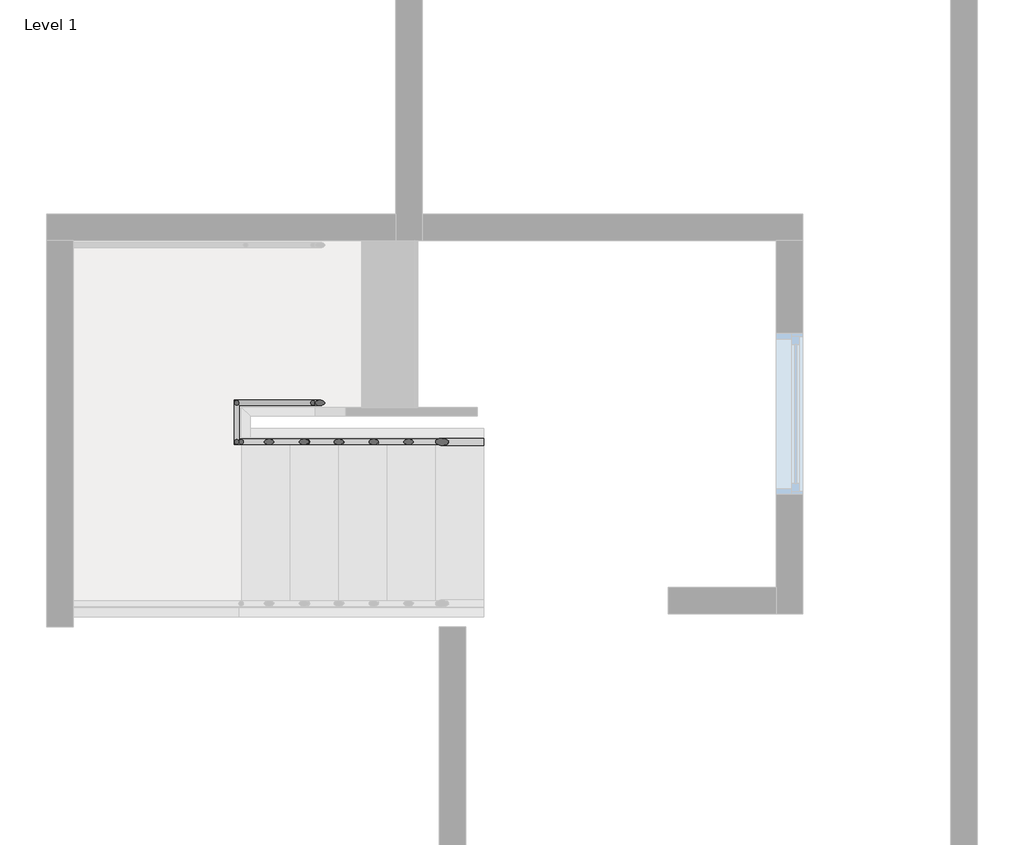
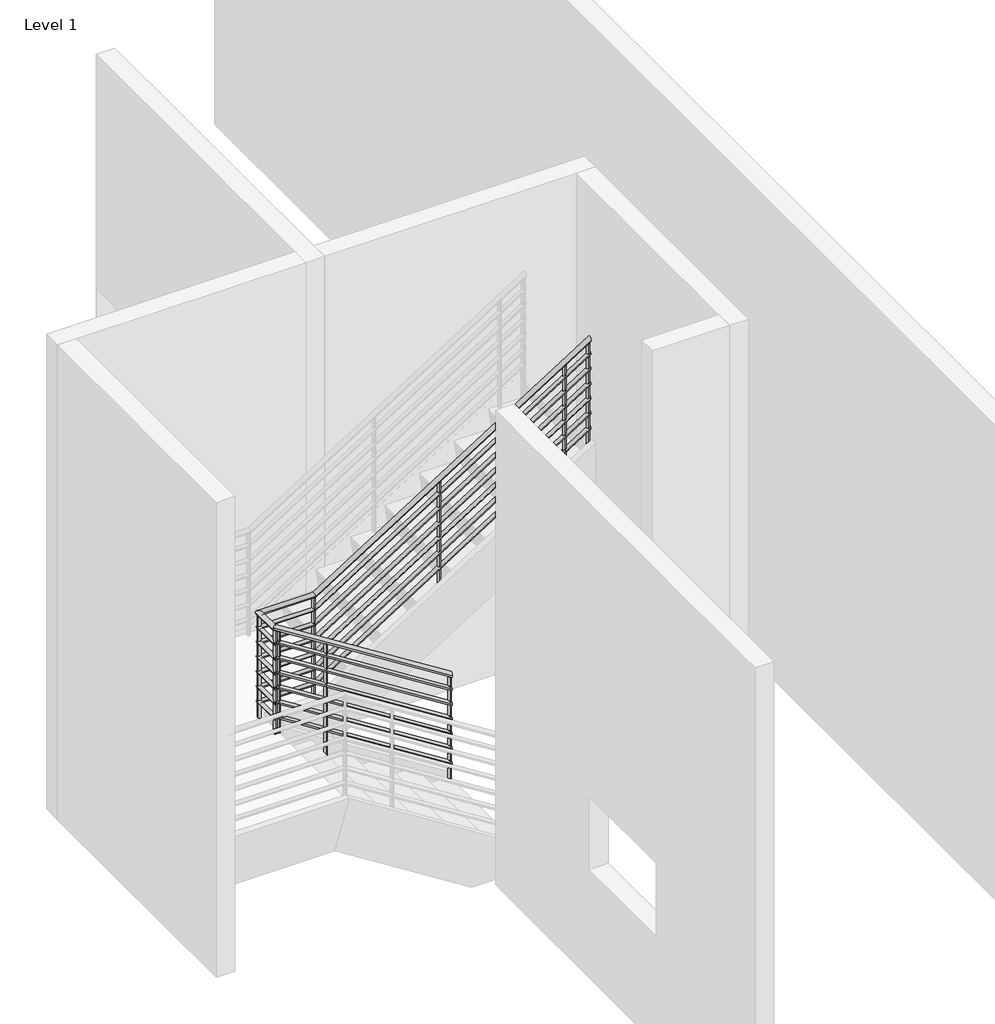
# One storey, part 3 of 4: 1 railing.
"""IFC4 building model written with IfcOpenShell, lengths in millimetres."""

from ifc_helpers import new_model, si_unit, point, frame, frame_2d, origin, place, context, project, spatial, circle_curve, ellipse_curve, trimmed, segment, composite_curve, outline, extrude, element, save
from ifc_brep_helpers import plane_surface, cylinder_surface, advanced_brep

model = new_model("IFC4")

# Units and contexts
model_context = context("Model", 3, world=origin())
ifc_project = project(units=[si_unit("LENGTHUNIT", "METRE", prefix="MILLI")], contexts=[model_context])

# Site, building, storey
site = spatial("IfcSite", under=ifc_project)
building = spatial("IfcBuilding", under=site)
storey = spatial("IfcBuildingStorey", under=building, Name="Level 1", Elevation=0.0)

# Railing
placement = place(None, origin())
element("IfcRailing", 1, ObjectType="900mm Pipe", at=placement, inside=storey, context=model_context, shape_type="SolidModel", body=[
    advanced_brep(
    [(-539.0915237, 1805.4567276, 1050.2491997), (-539.0915237, 1765.4567276, 1050.2491997), (-1933.2780119, 1805.4567276, 1931.9481645), (-1967.0848612, 1765.4567276, 1953.3279902)],
    [
        (0, 1, ellipse_curve(frame((-539.0915237, 1785.4567276, 1050.2491997), z_axis=(1.0, 0.0, 0.0), x_axis=(0.0, 0.0, -1.0)), 23.6638438, 20.0)),
        (1, 0, ellipse_curve(frame((-539.0915237, 1785.4567276, 1050.2491997), z_axis=(1.0, 0.0, 0.0), x_axis=(0.0, 0.0, -1.0)), 23.6638438, 20.0)),
        (2, 3, ellipse_curve(frame((-1950.1814365, 1785.4567276, 1942.6380773), z_axis=(-0.5976263089853376, 0.7071067811865505, 0.37794549184843795), x_axis=(0.597626308985345, 0.7071067811865448, -0.37794549184843707)), 28.2842712, 20.0)),
        (3, 2, ellipse_curve(frame((-1950.1814365, 1785.4567276, 1942.6380773), z_axis=(-0.5976263089853376, 0.7071067811865505, 0.37794549184843795), x_axis=(0.597626308985345, 0.7071067811865448, -0.37794549184843707)), 28.2842712, 20.0)),
        (0, 2),
        (3, 1),
    ],
    [
        plane_surface(frame((-539.0915237, 1785.4567276, 1073.9130435), z_axis=(1.0, 0.0, 0.0), x_axis=(0.0, -1.0, 0.0))),
        plane_surface(frame((-1939.4915237, 1785.4567276, 1959.541502), z_axis=(-0.5976263089853376, 0.7071067811865505, 0.37794549184843795), x_axis=(0.8017747781070204, 0.5270627453469413, 0.281712739610376))),
        cylinder_surface(frame((-549.7814365, 1785.4567276, 1057.0096189), z_axis=(0.8451712313980436, 0.0, -0.5344956404098304), x_axis=(0.0, -1.0, 0.0)), 20.0),
    ],
    [
        (0, [[1, 2]]),
        (1, [[3, 4]]),
        (2, [[-1, 5, -4, 6]]),
        (2, [[-2, -6, -3, -5]]),
    ],
),
    advanced_brep(
    [(-1919.4915237, 1813.050065, 1923.4782609), (-1959.4915237, 1779.2432158, 1923.4782609), (-1919.4915237, 1986.3593033, 1923.4782609), (-1959.4915237, 2026.3593033, 1923.4782609), (-1501.6762623, 1986.3593033, 1923.4782609), (-1501.6762623, 2026.3593033, 1923.4782609), (692.5302847, 1986.3593033, 3311.1187649), (692.5302847, 2026.3593033, 3311.1187649)],
    [
        (0, 1, ellipse_curve(frame((-1939.4915237, 1796.1466404, 1923.4782609), z_axis=(0.5976263089853376, -0.7071067811865505, -0.37794549184843795), x_axis=(-0.5976263089853452, -0.7071067811865446, 0.37794549184843695)), 28.2842712, 20.0)),
        (1, 0, ellipse_curve(frame((-1939.4915237, 1796.1466404, 1923.4782609), z_axis=(0.5976263089853376, -0.7071067811865505, -0.37794549184843795), x_axis=(-0.5976263089853452, -0.7071067811865446, 0.37794549184843695)), 28.2842712, 20.0)),
        (0, 2),
        (2, 3, ellipse_curve(frame((-1939.4915237, 2006.3593033, 1923.4782609), z_axis=(-0.7071067811865511, -0.707106781186544, 0.0), x_axis=(0.7071067811865441, -0.707106781186551, 0.0)), 28.2842712, 20.0)),
        (3, 1),
        (3, 2, ellipse_curve(frame((-1939.4915237, 2006.3593033, 1923.4782609), z_axis=(-0.7071067811865511, -0.707106781186544, 0.0), x_axis=(0.7071067811865441, -0.707106781186551, 0.0)), 28.2842712, 20.0)),
        (2, 4),
        (4, 5, ellipse_curve(frame((-1501.6762623, 2006.3593033, 1923.4782609), z_axis=(-0.9605132043335073, 0.0, -0.27823440531497556), x_axis=(-0.2782344053149757, 0.0, 0.9605132043335073)), 20.822202, 20.0)),
        (5, 3),
        (5, 4, ellipse_curve(frame((-1501.6762623, 2006.3593033, 1923.4782609), z_axis=(-0.9605132043335073, 0.0, -0.27823440531497556), x_axis=(-0.2782344053149757, 0.0, 0.9605132043335073)), 20.822202, 20.0)),
        (6, 7, ellipse_curve(frame((692.5302847, 2006.3593033, 3311.1187649), z_axis=(1.0, 0.0, 0.0), x_axis=(0.0, 0.0, -1.0)), 23.6638438, 20.0)),
        (7, 6, ellipse_curve(frame((692.5302847, 2006.3593033, 3311.1187649), z_axis=(1.0, 0.0, 0.0), x_axis=(0.0, 0.0, -1.0)), 23.6638438, 20.0)),
        (4, 6),
        (7, 5),
    ],
    [
        plane_surface(frame((-1939.4915237, 1785.4567276, 1943.4782609), z_axis=(0.5976263089853376, -0.7071067811865505, -0.37794549184843795), x_axis=(0.8017747781070204, 0.5270627453469413, 0.281712739610376))),
        cylinder_surface(frame((-1939.4915237, 1785.4567276, 1923.4782609), z_axis=(0.0, -1.0, 0.0), x_axis=(-1.0, 0.0, 0.0)), 20.0),
        cylinder_surface(frame((-1939.4915237, 2006.3593033, 1923.4782609), z_axis=(-1.0, 0.0, 0.0), x_axis=(0.0, 1.0, 0.0)), 20.0),
        plane_surface(frame((692.5302847, 2006.3593033, 3334.7826087), z_axis=(1.0, 0.0, 0.0), x_axis=(0.0, 1.0, 0.0))),
        cylinder_surface(frame((-1496.7798025, 2006.3593033, 1926.5748362), z_axis=(-0.8451712313980438, 0.0, -0.5344956404098301), x_axis=(0.0, 1.0, 0.0)), 20.0),
    ],
    [
        (0, [[1, 2]]),
        (1, [[-1, 3, 4, 5]]),
        (1, [[-2, -5, 6, -3]]),
        (2, [[-4, 7, 8, 9]]),
        (2, [[-6, -9, 10, -7]]),
        (3, [[11, 12]]),
        (4, [[-8, 13, -12, 14]]),
        (4, [[-10, -14, -11, -13]]),
    ],
),
    advanced_brep(
    [(-539.0915237, 1770.4567276, 931.1651606), (-539.0915237, 1800.4567276, 931.1651606), (-1918.4366135, 1770.4567276, 1803.4782609), (-1918.4366135, 1800.4567276, 1803.4782609), (-1954.4915237, 1770.4567276, 1803.4782609), (-1924.4915237, 1800.4567276, 1803.4782609), (-1954.4915237, 2021.3593033, 1803.4782609), (-1924.4915237, 1991.3593033, 1803.4782609), (-1503.1246256, 2021.3593033, 1803.4782609), (-1503.1246256, 1991.3593033, 1803.4782609), (692.5302847, 2021.3593033, 3192.0347258), (692.5302847, 1991.3593033, 3192.0347258)],
    [
        (0, 1, ellipse_curve(frame((-539.0915237, 1785.4567276, 931.1651606), z_axis=(1.0, 0.0, 0.0), x_axis=(0.0, 0.0, -1.0)), 17.7478828, 15.0)),
        (1, 0, ellipse_curve(frame((-539.0915237, 1785.4567276, 931.1651606), z_axis=(1.0, 0.0, 0.0), x_axis=(0.0, 0.0, -1.0)), 17.7478828, 15.0)),
        (0, 2),
        (2, 3, ellipse_curve(frame((-1918.4366135, 1785.4567276, 1803.4782609), z_axis=(0.9605132043335073, 0.0, -0.27823440531497584), x_axis=(-0.2782344053149764, 0.0, -0.9605132043335071)), 15.6166515, 15.0)),
        (3, 1),
        (3, 2, ellipse_curve(frame((-1918.4366135, 1785.4567276, 1803.4782609), z_axis=(0.9605132043335073, 0.0, -0.27823440531497584), x_axis=(-0.2782344053149764, 0.0, -0.9605132043335071)), 15.6166515, 15.0)),
        (2, 4),
        (4, 5, ellipse_curve(frame((-1939.4915237, 1785.4567276, 1803.4782609), z_axis=(0.7071067811865441, -0.7071067811865509, 0.0), x_axis=(0.707106781186551, 0.7071067811865441, 0.0)), 21.2132034, 15.0)),
        (5, 3),
        (5, 4, ellipse_curve(frame((-1939.4915237, 1785.4567276, 1803.4782609), z_axis=(0.7071067811865441, -0.7071067811865509, 0.0), x_axis=(0.707106781186551, 0.7071067811865441, 0.0)), 21.2132034, 15.0)),
        (4, 6),
        (6, 7, ellipse_curve(frame((-1939.4915237, 2006.3593033, 1803.4782609), z_axis=(-0.7071067811865511, -0.707106781186544, 0.0), x_axis=(0.7071067811865441, -0.707106781186551, 0.0)), 21.2132034, 15.0)),
        (7, 5),
        (7, 6, ellipse_curve(frame((-1939.4915237, 2006.3593033, 1803.4782609), z_axis=(-0.7071067811865511, -0.707106781186544, 0.0), x_axis=(0.7071067811865441, -0.707106781186551, 0.0)), 21.2132034, 15.0)),
        (6, 8),
        (8, 9, ellipse_curve(frame((-1503.1246256, 2006.3593033, 1803.4782609), z_axis=(-0.9605132043335072, 0.0, -0.2782344053149756), x_axis=(-0.27823440531497606, 0.0, 0.9605132043335073)), 15.6166515, 15.0)),
        (9, 7),
        (9, 8, ellipse_curve(frame((-1503.1246256, 2006.3593033, 1803.4782609), z_axis=(-0.9605132043335072, 0.0, -0.2782344053149756), x_axis=(-0.27823440531497606, 0.0, 0.9605132043335073)), 15.6166515, 15.0)),
        (10, 11, ellipse_curve(frame((692.5302847, 2006.3593033, 3192.0347258), z_axis=(1.0, 0.0, 0.0), x_axis=(0.0, 0.0, -1.0)), 17.7478828, 15.0)),
        (11, 10, ellipse_curve(frame((692.5302847, 2006.3593033, 3192.0347258), z_axis=(1.0, 0.0, 0.0), x_axis=(0.0, 0.0, -1.0)), 17.7478828, 15.0)),
        (8, 10),
        (11, 9),
    ],
    [
        plane_surface(frame((-539.0915237, 1785.4567276, 948.9130435), z_axis=(1.0, 0.0, 0.0), x_axis=(0.0, -1.0, 0.0))),
        cylinder_surface(frame((-547.1089583, 1785.4567276, 936.235475), z_axis=(0.8451712313980436, 0.0, -0.5344956404098303), x_axis=(0.0, 1.0, 0.0)), 15.0),
        cylinder_surface(frame((-1914.0915237, 1785.4567276, 1803.4782609), z_axis=(1.0, 0.0, 0.0), x_axis=(0.0, 1.0, 0.0)), 15.0),
        cylinder_surface(frame((-1939.4915237, 1785.4567276, 1803.4782609), z_axis=(0.0, -1.0, 0.0), x_axis=(1.0, 0.0, 0.0)), 15.0),
        cylinder_surface(frame((-1939.4915237, 2006.3593033, 1803.4782609), z_axis=(-1.0, 0.0, 0.0), x_axis=(0.0, -1.0, 0.0)), 15.0),
        plane_surface(frame((692.5302847, 2006.3593033, 3209.7826087), z_axis=(1.0, 0.0, 0.0), x_axis=(0.0, 1.0, 0.0))),
        cylinder_surface(frame((-1499.4522807, 2006.3593033, 1805.8006924), z_axis=(-0.8451712313980437, 0.0, -0.5344956404098301), x_axis=(0.0, -1.0, 0.0)), 15.0),
    ],
    [
        (0, [[1, 2]]),
        (1, [[-1, 3, 4, 5]]),
        (1, [[-2, -5, 6, -3]]),
        (2, [[-4, 7, 8, 9]]),
        (2, [[-6, -9, 10, -7]]),
        (3, [[-8, 11, 12, 13]]),
        (3, [[-10, -13, 14, -11]]),
        (4, [[-12, 15, 16, 17]]),
        (4, [[-14, -17, 18, -15]]),
        (5, [[19, 20]]),
        (6, [[-16, 21, -20, 22]]),
        (6, [[-18, -22, -19, -21]]),
    ],
),
    advanced_brep(
    [(-539.0915237, 1770.4567276, 806.1651606), (-539.0915237, 1800.4567276, 806.1651606), (-1918.4366135, 1770.4567276, 1678.4782609), (-1918.4366135, 1800.4567276, 1678.4782609), (-1954.4915237, 1770.4567276, 1678.4782609), (-1924.4915237, 1800.4567276, 1678.4782609), (-1954.4915237, 2021.3593033, 1678.4782609), (-1924.4915237, 1991.3593033, 1678.4782609), (-1503.1246256, 2021.3593033, 1678.4782609), (-1503.1246256, 1991.3593033, 1678.4782609), (692.5302847, 2021.3593033, 3067.0347258), (692.5302847, 1991.3593033, 3067.0347258)],
    [
        (0, 1, ellipse_curve(frame((-539.0915237, 1785.4567276, 806.1651606), z_axis=(1.0, 0.0, 0.0), x_axis=(0.0, 0.0, -1.0)), 17.7478828, 15.0)),
        (1, 0, ellipse_curve(frame((-539.0915237, 1785.4567276, 806.1651606), z_axis=(1.0, 0.0, 0.0), x_axis=(0.0, 0.0, -1.0)), 17.7478828, 15.0)),
        (0, 2),
        (2, 3, ellipse_curve(frame((-1918.4366135, 1785.4567276, 1678.4782609), z_axis=(0.9605132043335073, 0.0, -0.27823440531497584), x_axis=(-0.2782344053149764, 0.0, -0.9605132043335071)), 15.6166515, 15.0)),
        (3, 1),
        (3, 2, ellipse_curve(frame((-1918.4366135, 1785.4567276, 1678.4782609), z_axis=(0.9605132043335073, 0.0, -0.27823440531497584), x_axis=(-0.2782344053149764, 0.0, -0.9605132043335071)), 15.6166515, 15.0)),
        (2, 4),
        (4, 5, ellipse_curve(frame((-1939.4915237, 1785.4567276, 1678.4782609), z_axis=(0.7071067811865441, -0.7071067811865509, 0.0), x_axis=(0.707106781186551, 0.7071067811865441, 0.0)), 21.2132034, 15.0)),
        (5, 3),
        (5, 4, ellipse_curve(frame((-1939.4915237, 1785.4567276, 1678.4782609), z_axis=(0.7071067811865441, -0.7071067811865509, 0.0), x_axis=(0.707106781186551, 0.7071067811865441, 0.0)), 21.2132034, 15.0)),
        (4, 6),
        (6, 7, ellipse_curve(frame((-1939.4915237, 2006.3593033, 1678.4782609), z_axis=(-0.7071067811865511, -0.707106781186544, 0.0), x_axis=(0.7071067811865441, -0.707106781186551, 0.0)), 21.2132034, 15.0)),
        (7, 5),
        (7, 6, ellipse_curve(frame((-1939.4915237, 2006.3593033, 1678.4782609), z_axis=(-0.7071067811865511, -0.707106781186544, 0.0), x_axis=(0.7071067811865441, -0.707106781186551, 0.0)), 21.2132034, 15.0)),
        (6, 8),
        (8, 9, ellipse_curve(frame((-1503.1246256, 2006.3593033, 1678.4782609), z_axis=(-0.9605132043335073, 0.0, -0.2782344053149756), x_axis=(-0.2782344053149757, 0.0, 0.9605132043335073)), 15.6166515, 15.0)),
        (9, 7),
        (9, 8, ellipse_curve(frame((-1503.1246256, 2006.3593033, 1678.4782609), z_axis=(-0.9605132043335073, 0.0, -0.2782344053149756), x_axis=(-0.2782344053149757, 0.0, 0.9605132043335073)), 15.6166515, 15.0)),
        (10, 11, ellipse_curve(frame((692.5302847, 2006.3593033, 3067.0347258), z_axis=(1.0, 0.0, 0.0), x_axis=(0.0, 0.0, -1.0)), 17.7478828, 15.0)),
        (11, 10, ellipse_curve(frame((692.5302847, 2006.3593033, 3067.0347258), z_axis=(1.0, 0.0, 0.0), x_axis=(0.0, 0.0, -1.0)), 17.7478828, 15.0)),
        (8, 10),
        (11, 9),
    ],
    [
        plane_surface(frame((-539.0915237, 1785.4567276, 823.9130435), z_axis=(1.0, 0.0, 0.0), x_axis=(0.0, -1.0, 0.0))),
        cylinder_surface(frame((-547.1089583, 1785.4567276, 811.235475), z_axis=(0.8451712313980436, 0.0, -0.5344956404098303), x_axis=(0.0, 1.0, 0.0)), 15.0),
        cylinder_surface(frame((-1914.0915237, 1785.4567276, 1678.4782609), z_axis=(1.0, 0.0, 0.0), x_axis=(0.0, 1.0, 0.0)), 15.0),
        cylinder_surface(frame((-1939.4915237, 1785.4567276, 1678.4782609), z_axis=(0.0, -1.0, 0.0), x_axis=(1.0, 0.0, 0.0)), 15.0),
        cylinder_surface(frame((-1939.4915237, 2006.3593033, 1678.4782609), z_axis=(-1.0, 0.0, 0.0), x_axis=(0.0, -1.0, 0.0)), 15.0),
        plane_surface(frame((692.5302847, 2006.3593033, 3084.7826087), z_axis=(1.0, 0.0, 0.0), x_axis=(0.0, 1.0, 0.0))),
        cylinder_surface(frame((-1499.4522807, 2006.3593033, 1680.8006924), z_axis=(-0.8451712313980438, 0.0, -0.5344956404098301), x_axis=(0.0, -1.0, 0.0)), 15.0),
    ],
    [
        (0, [[1, 2]]),
        (1, [[-1, 3, 4, 5]]),
        (1, [[-2, -5, 6, -3]]),
        (2, [[-4, 7, 8, 9]]),
        (2, [[-6, -9, 10, -7]]),
        (3, [[-8, 11, 12, 13]]),
        (3, [[-10, -13, 14, -11]]),
        (4, [[-12, 15, 16, 17]]),
        (4, [[-14, -17, 18, -15]]),
        (5, [[19, 20]]),
        (6, [[-16, 21, -20, 22]]),
        (6, [[-18, -22, -19, -21]]),
    ],
),
    advanced_brep(
    [(-539.0915237, 1770.4567276, 681.1651606), (-539.0915237, 1800.4567276, 681.1651606), (-1918.4366135, 1770.4567276, 1553.4782609), (-1918.4366135, 1800.4567276, 1553.4782609), (-1954.4915237, 1770.4567276, 1553.4782609), (-1924.4915237, 1800.4567276, 1553.4782609), (-1954.4915237, 2021.3593033, 1553.4782609), (-1924.4915237, 1991.3593033, 1553.4782609), (-1503.1246256, 2021.3593033, 1553.4782609), (-1503.1246256, 1991.3593033, 1553.4782609), (692.5302847, 2021.3593033, 2942.0347258), (692.5302847, 1991.3593033, 2942.0347258)],
    [
        (0, 1, ellipse_curve(frame((-539.0915237, 1785.4567276, 681.1651606), z_axis=(1.0, 0.0, 0.0), x_axis=(0.0, 0.0, -1.0)), 17.7478828, 15.0)),
        (1, 0, ellipse_curve(frame((-539.0915237, 1785.4567276, 681.1651606), z_axis=(1.0, 0.0, 0.0), x_axis=(0.0, 0.0, -1.0)), 17.7478828, 15.0)),
        (0, 2),
        (2, 3, ellipse_curve(frame((-1918.4366135, 1785.4567276, 1553.4782609), z_axis=(0.9605132043335073, 0.0, -0.27823440531497584), x_axis=(-0.2782344053149764, 0.0, -0.9605132043335071)), 15.6166515, 15.0)),
        (3, 1),
        (3, 2, ellipse_curve(frame((-1918.4366135, 1785.4567276, 1553.4782609), z_axis=(0.9605132043335073, 0.0, -0.27823440531497584), x_axis=(-0.2782344053149764, 0.0, -0.9605132043335071)), 15.6166515, 15.0)),
        (2, 4),
        (4, 5, ellipse_curve(frame((-1939.4915237, 1785.4567276, 1553.4782609), z_axis=(0.7071067811865441, -0.7071067811865509, 0.0), x_axis=(0.707106781186551, 0.7071067811865441, 0.0)), 21.2132034, 15.0)),
        (5, 3),
        (5, 4, ellipse_curve(frame((-1939.4915237, 1785.4567276, 1553.4782609), z_axis=(0.7071067811865441, -0.7071067811865509, 0.0), x_axis=(0.707106781186551, 0.7071067811865441, 0.0)), 21.2132034, 15.0)),
        (4, 6),
        (6, 7, ellipse_curve(frame((-1939.4915237, 2006.3593033, 1553.4782609), z_axis=(-0.7071067811865511, -0.707106781186544, 0.0), x_axis=(0.7071067811865441, -0.707106781186551, 0.0)), 21.2132034, 15.0)),
        (7, 5),
        (7, 6, ellipse_curve(frame((-1939.4915237, 2006.3593033, 1553.4782609), z_axis=(-0.7071067811865511, -0.707106781186544, 0.0), x_axis=(0.7071067811865441, -0.707106781186551, 0.0)), 21.2132034, 15.0)),
        (6, 8),
        (8, 9, ellipse_curve(frame((-1503.1246256, 2006.3593033, 1553.4782609), z_axis=(-0.9605132043335073, 0.0, -0.2782344053149756), x_axis=(-0.2782344053149757, 0.0, 0.9605132043335073)), 15.6166515, 15.0)),
        (9, 7),
        (9, 8, ellipse_curve(frame((-1503.1246256, 2006.3593033, 1553.4782609), z_axis=(-0.9605132043335073, 0.0, -0.2782344053149756), x_axis=(-0.2782344053149757, 0.0, 0.9605132043335073)), 15.6166515, 15.0)),
        (10, 11, ellipse_curve(frame((692.5302847, 2006.3593033, 2942.0347258), z_axis=(1.0, 0.0, 0.0), x_axis=(0.0, 0.0, -1.0)), 17.7478828, 15.0)),
        (11, 10, ellipse_curve(frame((692.5302847, 2006.3593033, 2942.0347258), z_axis=(1.0, 0.0, 0.0), x_axis=(0.0, 0.0, -1.0)), 17.7478828, 15.0)),
        (8, 10),
        (11, 9),
    ],
    [
        plane_surface(frame((-539.0915237, 1785.4567276, 698.9130435), z_axis=(1.0, 0.0, 0.0), x_axis=(0.0, -1.0, 0.0))),
        cylinder_surface(frame((-547.1089583, 1785.4567276, 686.235475), z_axis=(0.8451712313980436, 0.0, -0.5344956404098303), x_axis=(0.0, 1.0, 0.0)), 15.0),
        cylinder_surface(frame((-1914.0915237, 1785.4567276, 1553.4782609), z_axis=(1.0, 0.0, 0.0), x_axis=(0.0, 1.0, 0.0)), 15.0),
        cylinder_surface(frame((-1939.4915237, 1785.4567276, 1553.4782609), z_axis=(0.0, -1.0, 0.0), x_axis=(1.0, 0.0, 0.0)), 15.0),
        cylinder_surface(frame((-1939.4915237, 2006.3593033, 1553.4782609), z_axis=(-1.0, 0.0, 0.0), x_axis=(0.0, -1.0, 0.0)), 15.0),
        plane_surface(frame((692.5302847, 2006.3593033, 2959.7826087), z_axis=(1.0, 0.0, 0.0), x_axis=(0.0, 1.0, 0.0))),
        cylinder_surface(frame((-1499.4522807, 2006.3593033, 1555.8006924), z_axis=(-0.8451712313980438, 0.0, -0.5344956404098301), x_axis=(0.0, -1.0, 0.0)), 15.0),
    ],
    [
        (0, [[1, 2]]),
        (1, [[-1, 3, 4, 5]]),
        (1, [[-2, -5, 6, -3]]),
        (2, [[-4, 7, 8, 9]]),
        (2, [[-6, -9, 10, -7]]),
        (3, [[-8, 11, 12, 13]]),
        (3, [[-10, -13, 14, -11]]),
        (4, [[-12, 15, 16, 17]]),
        (4, [[-14, -17, 18, -15]]),
        (5, [[19, 20]]),
        (6, [[-16, 21, -20, 22]]),
        (6, [[-18, -22, -19, -21]]),
    ],
),
    advanced_brep(
    [(-539.0915237, 1770.4567276, 556.1651606), (-539.0915237, 1800.4567276, 556.1651606), (-1918.4366135, 1770.4567276, 1428.4782609), (-1918.4366135, 1800.4567276, 1428.4782609), (-1954.4915237, 1770.4567276, 1428.4782609), (-1924.4915237, 1800.4567276, 1428.4782609), (-1954.4915237, 2021.3593033, 1428.4782609), (-1924.4915237, 1991.3593033, 1428.4782609), (-1503.1246256, 2021.3593033, 1428.4782609), (-1503.1246256, 1991.3593033, 1428.4782609), (692.5302847, 2021.3593033, 2817.0347258), (692.5302847, 1991.3593033, 2817.0347258)],
    [
        (0, 1, ellipse_curve(frame((-539.0915237, 1785.4567276, 556.1651606), z_axis=(1.0, 0.0, 0.0), x_axis=(0.0, 0.0, -1.0)), 17.7478828, 15.0)),
        (1, 0, ellipse_curve(frame((-539.0915237, 1785.4567276, 556.1651606), z_axis=(1.0, 0.0, 0.0), x_axis=(0.0, 0.0, -1.0)), 17.7478828, 15.0)),
        (0, 2),
        (2, 3, ellipse_curve(frame((-1918.4366135, 1785.4567276, 1428.4782609), z_axis=(0.9605132043335073, 0.0, -0.27823440531497584), x_axis=(-0.2782344053149764, 0.0, -0.9605132043335071)), 15.6166515, 15.0)),
        (3, 1),
        (3, 2, ellipse_curve(frame((-1918.4366135, 1785.4567276, 1428.4782609), z_axis=(0.9605132043335073, 0.0, -0.27823440531497584), x_axis=(-0.2782344053149764, 0.0, -0.9605132043335071)), 15.6166515, 15.0)),
        (2, 4),
        (4, 5, ellipse_curve(frame((-1939.4915237, 1785.4567276, 1428.4782609), z_axis=(0.7071067811865441, -0.7071067811865509, 0.0), x_axis=(0.707106781186551, 0.7071067811865441, 0.0)), 21.2132034, 15.0)),
        (5, 3),
        (5, 4, ellipse_curve(frame((-1939.4915237, 1785.4567276, 1428.4782609), z_axis=(0.7071067811865441, -0.7071067811865509, 0.0), x_axis=(0.707106781186551, 0.7071067811865441, 0.0)), 21.2132034, 15.0)),
        (4, 6),
        (6, 7, ellipse_curve(frame((-1939.4915237, 2006.3593033, 1428.4782609), z_axis=(-0.7071067811865511, -0.707106781186544, 0.0), x_axis=(0.7071067811865441, -0.707106781186551, 0.0)), 21.2132034, 15.0)),
        (7, 5),
        (7, 6, ellipse_curve(frame((-1939.4915237, 2006.3593033, 1428.4782609), z_axis=(-0.7071067811865511, -0.707106781186544, 0.0), x_axis=(0.7071067811865441, -0.707106781186551, 0.0)), 21.2132034, 15.0)),
        (6, 8),
        (8, 9, ellipse_curve(frame((-1503.1246256, 2006.3593033, 1428.4782609), z_axis=(-0.9605132043335073, 0.0, -0.2782344053149756), x_axis=(-0.2782344053149757, 0.0, 0.9605132043335073)), 15.6166515, 15.0)),
        (9, 7),
        (9, 8, ellipse_curve(frame((-1503.1246256, 2006.3593033, 1428.4782609), z_axis=(-0.9605132043335073, 0.0, -0.2782344053149756), x_axis=(-0.2782344053149757, 0.0, 0.9605132043335073)), 15.6166515, 15.0)),
        (10, 11, ellipse_curve(frame((692.5302847, 2006.3593033, 2817.0347258), z_axis=(1.0, 0.0, 0.0), x_axis=(0.0, 0.0, -1.0)), 17.7478828, 15.0)),
        (11, 10, ellipse_curve(frame((692.5302847, 2006.3593033, 2817.0347258), z_axis=(1.0, 0.0, 0.0), x_axis=(0.0, 0.0, -1.0)), 17.7478828, 15.0)),
        (8, 10),
        (11, 9),
    ],
    [
        plane_surface(frame((-539.0915237, 1785.4567276, 573.9130435), z_axis=(1.0, 0.0, 0.0), x_axis=(0.0, -1.0, 0.0))),
        cylinder_surface(frame((-547.1089583, 1785.4567276, 561.235475), z_axis=(0.8451712313980436, 0.0, -0.5344956404098303), x_axis=(0.0, 1.0, 0.0)), 15.0),
        cylinder_surface(frame((-1914.0915237, 1785.4567276, 1428.4782609), z_axis=(1.0, 0.0, 0.0), x_axis=(0.0, 1.0, 0.0)), 15.0),
        cylinder_surface(frame((-1939.4915237, 1785.4567276, 1428.4782609), z_axis=(0.0, -1.0, 0.0), x_axis=(1.0, 0.0, 0.0)), 15.0),
        cylinder_surface(frame((-1939.4915237, 2006.3593033, 1428.4782609), z_axis=(-1.0, 0.0, 0.0), x_axis=(0.0, -1.0, 0.0)), 15.0),
        plane_surface(frame((692.5302847, 2006.3593033, 2834.7826087), z_axis=(1.0, 0.0, 0.0), x_axis=(0.0, 1.0, 0.0))),
        cylinder_surface(frame((-1499.4522807, 2006.3593033, 1430.8006924), z_axis=(-0.8451712313980438, 0.0, -0.5344956404098301), x_axis=(0.0, -1.0, 0.0)), 15.0),
    ],
    [
        (0, [[1, 2]]),
        (1, [[-1, 3, 4, 5]]),
        (1, [[-2, -5, 6, -3]]),
        (2, [[-4, 7, 8, 9]]),
        (2, [[-6, -9, 10, -7]]),
        (3, [[-8, 11, 12, 13]]),
        (3, [[-10, -13, 14, -11]]),
        (4, [[-12, 15, 16, 17]]),
        (4, [[-14, -17, 18, -15]]),
        (5, [[19, 20]]),
        (6, [[-16, 21, -20, 22]]),
        (6, [[-18, -22, -19, -21]]),
    ],
),
    advanced_brep(
    [(-539.0915237, 1770.4567276, 431.1651606), (-539.0915237, 1800.4567276, 431.1651606), (-1918.4366135, 1770.4567276, 1303.4782609), (-1918.4366135, 1800.4567276, 1303.4782609), (-1954.4915237, 1770.4567276, 1303.4782609), (-1924.4915237, 1800.4567276, 1303.4782609), (-1954.4915237, 2021.3593033, 1303.4782609), (-1924.4915237, 1991.3593033, 1303.4782609), (-1503.1246256, 2021.3593033, 1303.4782609), (-1503.1246256, 1991.3593033, 1303.4782609), (692.5302847, 2021.3593033, 2692.0347258), (692.5302847, 1991.3593033, 2692.0347258)],
    [
        (0, 1, ellipse_curve(frame((-539.0915237, 1785.4567276, 431.1651606), z_axis=(1.0, 0.0, 0.0), x_axis=(0.0, 0.0, -1.0)), 17.7478828, 15.0)),
        (1, 0, ellipse_curve(frame((-539.0915237, 1785.4567276, 431.1651606), z_axis=(1.0, 0.0, 0.0), x_axis=(0.0, 0.0, -1.0)), 17.7478828, 15.0)),
        (0, 2),
        (2, 3, ellipse_curve(frame((-1918.4366135, 1785.4567276, 1303.4782609), z_axis=(0.9605132043335073, 0.0, -0.27823440531497584), x_axis=(-0.2782344053149764, 0.0, -0.9605132043335071)), 15.6166515, 15.0)),
        (3, 1),
        (3, 2, ellipse_curve(frame((-1918.4366135, 1785.4567276, 1303.4782609), z_axis=(0.9605132043335073, 0.0, -0.27823440531497584), x_axis=(-0.2782344053149764, 0.0, -0.9605132043335071)), 15.6166515, 15.0)),
        (2, 4),
        (4, 5, ellipse_curve(frame((-1939.4915237, 1785.4567276, 1303.4782609), z_axis=(0.7071067811865441, -0.7071067811865509, 0.0), x_axis=(0.707106781186551, 0.7071067811865441, 0.0)), 21.2132034, 15.0)),
        (5, 3),
        (5, 4, ellipse_curve(frame((-1939.4915237, 1785.4567276, 1303.4782609), z_axis=(0.7071067811865441, -0.7071067811865509, 0.0), x_axis=(0.707106781186551, 0.7071067811865441, 0.0)), 21.2132034, 15.0)),
        (4, 6),
        (6, 7, ellipse_curve(frame((-1939.4915237, 2006.3593033, 1303.4782609), z_axis=(-0.7071067811865511, -0.707106781186544, 0.0), x_axis=(0.7071067811865441, -0.707106781186551, 0.0)), 21.2132034, 15.0)),
        (7, 5),
        (7, 6, ellipse_curve(frame((-1939.4915237, 2006.3593033, 1303.4782609), z_axis=(-0.7071067811865511, -0.707106781186544, 0.0), x_axis=(0.7071067811865441, -0.707106781186551, 0.0)), 21.2132034, 15.0)),
        (6, 8),
        (8, 9, ellipse_curve(frame((-1503.1246256, 2006.3593033, 1303.4782609), z_axis=(-0.9605132043335072, 0.0, -0.2782344053149756), x_axis=(-0.27823440531497606, 0.0, 0.9605132043335073)), 15.6166515, 15.0)),
        (9, 7),
        (9, 8, ellipse_curve(frame((-1503.1246256, 2006.3593033, 1303.4782609), z_axis=(-0.9605132043335072, 0.0, -0.2782344053149756), x_axis=(-0.27823440531497606, 0.0, 0.9605132043335073)), 15.6166515, 15.0)),
        (10, 11, ellipse_curve(frame((692.5302847, 2006.3593033, 2692.0347258), z_axis=(1.0, 0.0, 0.0), x_axis=(0.0, 0.0, -1.0)), 17.7478828, 15.0)),
        (11, 10, ellipse_curve(frame((692.5302847, 2006.3593033, 2692.0347258), z_axis=(1.0, 0.0, 0.0), x_axis=(0.0, 0.0, -1.0)), 17.7478828, 15.0)),
        (8, 10),
        (11, 9),
    ],
    [
        plane_surface(frame((-539.0915237, 1785.4567276, 448.9130435), z_axis=(1.0, 0.0, 0.0), x_axis=(0.0, -1.0, 0.0))),
        cylinder_surface(frame((-547.1089583, 1785.4567276, 436.235475), z_axis=(0.8451712313980436, 0.0, -0.5344956404098303), x_axis=(0.0, 1.0, 0.0)), 15.0),
        cylinder_surface(frame((-1914.0915237, 1785.4567276, 1303.4782609), z_axis=(1.0, 0.0, 0.0), x_axis=(0.0, 1.0, 0.0)), 15.0),
        cylinder_surface(frame((-1939.4915237, 1785.4567276, 1303.4782609), z_axis=(0.0, -1.0, 0.0), x_axis=(1.0, 0.0, 0.0)), 15.0),
        cylinder_surface(frame((-1939.4915237, 2006.3593033, 1303.4782609), z_axis=(-1.0, 0.0, 0.0), x_axis=(0.0, -1.0, 0.0)), 15.0),
        plane_surface(frame((692.5302847, 2006.3593033, 2709.7826087), z_axis=(1.0, 0.0, 0.0), x_axis=(0.0, 1.0, 0.0))),
        cylinder_surface(frame((-1499.4522807, 2006.3593033, 1305.8006924), z_axis=(-0.8451712313980437, 0.0, -0.5344956404098301), x_axis=(0.0, -1.0, 0.0)), 15.0),
    ],
    [
        (0, [[1, 2]]),
        (1, [[-1, 3, 4, 5]]),
        (1, [[-2, -5, 6, -3]]),
        (2, [[-4, 7, 8, 9]]),
        (2, [[-6, -9, 10, -7]]),
        (3, [[-8, 11, 12, 13]]),
        (3, [[-10, -13, 14, -11]]),
        (4, [[-12, 15, 16, 17]]),
        (4, [[-14, -17, 18, -15]]),
        (5, [[19, 20]]),
        (6, [[-16, 21, -20, 22]]),
        (6, [[-18, -22, -19, -21]]),
    ],
),
    advanced_brep(
    [(-539.0915237, 1770.4567276, 306.1651606), (-539.0915237, 1800.4567276, 306.1651606), (-1918.4366135, 1770.4567276, 1178.4782609), (-1918.4366135, 1800.4567276, 1178.4782609), (-1954.4915237, 1770.4567276, 1178.4782609), (-1924.4915237, 1800.4567276, 1178.4782609), (-1954.4915237, 2021.3593033, 1178.4782609), (-1924.4915237, 1991.3593033, 1178.4782609), (-1503.1246256, 2021.3593033, 1178.4782609), (-1503.1246256, 1991.3593033, 1178.4782609), (692.5302847, 2021.3593033, 2567.0347258), (692.5302847, 1991.3593033, 2567.0347258)],
    [
        (0, 1, ellipse_curve(frame((-539.0915237, 1785.4567276, 306.1651606), z_axis=(1.0, 0.0, 0.0), x_axis=(0.0, 0.0, -1.0)), 17.7478828, 15.0)),
        (1, 0, ellipse_curve(frame((-539.0915237, 1785.4567276, 306.1651606), z_axis=(1.0, 0.0, 0.0), x_axis=(0.0, 0.0, -1.0)), 17.7478828, 15.0)),
        (0, 2),
        (2, 3, ellipse_curve(frame((-1918.4366135, 1785.4567276, 1178.4782609), z_axis=(0.9605132043335073, 0.0, -0.27823440531497584), x_axis=(-0.2782344053149764, 0.0, -0.9605132043335071)), 15.6166515, 15.0)),
        (3, 1),
        (3, 2, ellipse_curve(frame((-1918.4366135, 1785.4567276, 1178.4782609), z_axis=(0.9605132043335073, 0.0, -0.27823440531497584), x_axis=(-0.2782344053149764, 0.0, -0.9605132043335071)), 15.6166515, 15.0)),
        (2, 4),
        (4, 5, ellipse_curve(frame((-1939.4915237, 1785.4567276, 1178.4782609), z_axis=(0.7071067811865441, -0.7071067811865509, 0.0), x_axis=(0.707106781186551, 0.7071067811865441, 0.0)), 21.2132034, 15.0)),
        (5, 3),
        (5, 4, ellipse_curve(frame((-1939.4915237, 1785.4567276, 1178.4782609), z_axis=(0.7071067811865441, -0.7071067811865509, 0.0), x_axis=(0.707106781186551, 0.7071067811865441, 0.0)), 21.2132034, 15.0)),
        (4, 6),
        (6, 7, ellipse_curve(frame((-1939.4915237, 2006.3593033, 1178.4782609), z_axis=(-0.7071067811865511, -0.707106781186544, 0.0), x_axis=(0.7071067811865441, -0.707106781186551, 0.0)), 21.2132034, 15.0)),
        (7, 5),
        (7, 6, ellipse_curve(frame((-1939.4915237, 2006.3593033, 1178.4782609), z_axis=(-0.7071067811865511, -0.707106781186544, 0.0), x_axis=(0.7071067811865441, -0.707106781186551, 0.0)), 21.2132034, 15.0)),
        (6, 8),
        (8, 9, ellipse_curve(frame((-1503.1246256, 2006.3593033, 1178.4782609), z_axis=(-0.9605132043335073, 0.0, -0.2782344053149756), x_axis=(-0.2782344053149757, 0.0, 0.9605132043335073)), 15.6166515, 15.0)),
        (9, 7),
        (9, 8, ellipse_curve(frame((-1503.1246256, 2006.3593033, 1178.4782609), z_axis=(-0.9605132043335073, 0.0, -0.2782344053149756), x_axis=(-0.2782344053149757, 0.0, 0.9605132043335073)), 15.6166515, 15.0)),
        (10, 11, ellipse_curve(frame((692.5302847, 2006.3593033, 2567.0347258), z_axis=(1.0, 0.0, 0.0), x_axis=(0.0, 0.0, -1.0)), 17.7478828, 15.0)),
        (11, 10, ellipse_curve(frame((692.5302847, 2006.3593033, 2567.0347258), z_axis=(1.0, 0.0, 0.0), x_axis=(0.0, 0.0, -1.0)), 17.7478828, 15.0)),
        (8, 10),
        (11, 9),
    ],
    [
        plane_surface(frame((-539.0915237, 1785.4567276, 323.9130435), z_axis=(1.0, 0.0, 0.0), x_axis=(0.0, -1.0, 0.0))),
        cylinder_surface(frame((-547.1089583, 1785.4567276, 311.235475), z_axis=(0.8451712313980436, 0.0, -0.5344956404098303), x_axis=(0.0, 1.0, 0.0)), 15.0),
        cylinder_surface(frame((-1914.0915237, 1785.4567276, 1178.4782609), z_axis=(1.0, 0.0, 0.0), x_axis=(0.0, 1.0, 0.0)), 15.0),
        cylinder_surface(frame((-1939.4915237, 1785.4567276, 1178.4782609), z_axis=(0.0, -1.0, 0.0), x_axis=(1.0, 0.0, 0.0)), 15.0),
        cylinder_surface(frame((-1939.4915237, 2006.3593033, 1178.4782609), z_axis=(-1.0, 0.0, 0.0), x_axis=(0.0, -1.0, 0.0)), 15.0),
        plane_surface(frame((692.5302847, 2006.3593033, 2584.7826087), z_axis=(1.0, 0.0, 0.0), x_axis=(0.0, 1.0, 0.0))),
        cylinder_surface(frame((-1499.4522807, 2006.3593033, 1180.8006924), z_axis=(-0.8451712313980438, 0.0, -0.5344956404098301), x_axis=(0.0, -1.0, 0.0)), 15.0),
    ],
    [
        (0, [[1, 2]]),
        (1, [[-1, 3, 4, 5]]),
        (1, [[-2, -5, 6, -3]]),
        (2, [[-4, 7, 8, 9]]),
        (2, [[-6, -9, 10, -7]]),
        (3, [[-8, 11, 12, 13]]),
        (3, [[-10, -13, 14, -11]]),
        (4, [[-12, 15, 16, 17]]),
        (4, [[-14, -17, 18, -15]]),
        (5, [[19, 20]]),
        (6, [[-16, 21, -20, 22]]),
        (6, [[-18, -22, -19, -21]]),
    ],
),
    advanced_brep(
    [(492.5302847, 1993.8593033, 3160.9727077), (492.5302847, 1993.8593033, 2260.8695652), (492.5302847, 2018.8593033, 2260.8695652), (492.5302847, 2018.8593033, 3160.9727077)],
    [
        (0, 1),
        (1, 2, circle_curve(frame((492.5302847, 2006.3593033, 2260.8695652), z_axis=(0.0, 0.0, 1.0), x_axis=(0.0, 1.0, 0.0)), 12.5)),
        (2, 3),
        (3, 0, ellipse_curve(frame((492.5302847, 2006.3593033, 3160.9727077), z_axis=(0.5344956404098302, 0.0, -0.8451712313980437), x_axis=(0.8451712313980437, 0.0, 0.53449564040983)), 14.7899024, 12.5)),
        (0, 3, ellipse_curve(frame((492.5302847, 2006.3593033, 3160.9727077), z_axis=(0.5344956404098302, 0.0, -0.8451712313980437), x_axis=(0.8451712313980437, 0.0, 0.53449564040983)), 14.7899024, 12.5)),
        (2, 1, circle_curve(frame((492.5302847, 2006.3593033, 2260.8695652), z_axis=(0.0, 0.0, 1.0), x_axis=(0.0, 1.0, 0.0)), 12.5)),
    ],
    [
        cylinder_surface(frame((492.5302847, 2006.3593033, 2160.8695652), z_axis=(0.0, 0.0, 1.0), x_axis=(0.0, 1.0, 0.0)), 12.5),
        plane_surface(frame((517.5302847, 2031.3593033, 3176.7829843), z_axis=(-0.5344956404098302, 0.0, 0.8451712313980437), x_axis=(0.0, -1.0, 0.0))),
        plane_surface(frame((467.5302847, 2031.3593033, 2260.8695652), z_axis=(0.0, 0.0, -1.0), x_axis=(0.0, -1.0, 0.0))),
    ],
    [
        (0, [[1, 2, 3, 4]]),
        (0, [[-1, 5, -3, 6]]),
        (1, [[-4, -5]]),
        (2, [[-2, -6]]),
    ],
),
    advanced_brep(
    [(-507.4697153, 1993.8593033, 2528.5616405), (-507.4697153, 1993.8593033, 1565.2173913), (-507.4697153, 2018.8593033, 1565.2173913), (-507.4697153, 2018.8593033, 2528.5616405)],
    [
        (0, 1),
        (1, 2, circle_curve(frame((-507.4697153, 2006.3593033, 1565.2173913), z_axis=(0.0, 0.0, 1.0), x_axis=(0.0, 1.0, 0.0)), 12.5)),
        (2, 3),
        (3, 0, ellipse_curve(frame((-507.4697153, 2006.3593033, 2528.5616405), z_axis=(0.5344956404098302, 0.0, -0.8451712313980437), x_axis=(0.8451712313980437, 0.0, 0.53449564040983)), 14.7899024, 12.5)),
        (0, 3, ellipse_curve(frame((-507.4697153, 2006.3593033, 2528.5616405), z_axis=(0.5344956404098302, 0.0, -0.8451712313980437), x_axis=(0.8451712313980437, 0.0, 0.53449564040983)), 14.7899024, 12.5)),
        (2, 1, circle_curve(frame((-507.4697153, 2006.3593033, 1565.2173913), z_axis=(0.0, 0.0, 1.0), x_axis=(0.0, 1.0, 0.0)), 12.5)),
    ],
    [
        cylinder_surface(frame((-507.4697153, 2006.3593033, 1465.2173913), z_axis=(0.0, 0.0, 1.0), x_axis=(0.0, 1.0, 0.0)), 12.5),
        plane_surface(frame((-482.4697153, 2031.3593033, 2544.3719172), z_axis=(-0.5344956404098302, 0.0, 0.8451712313980437), x_axis=(0.0, -1.0, 0.0))),
        plane_surface(frame((-532.4697153, 2031.3593033, 1565.2173913), z_axis=(0.0, 0.0, -1.0), x_axis=(0.0, -1.0, 0.0))),
    ],
    [
        (0, [[1, 2, 3, 4]]),
        (0, [[-1, 5, -3, 6]]),
        (1, [[-4, -5]]),
        (2, [[-2, -6]]),
    ],
),
    advanced_brep(
    [(-1539.0915237, 1797.9567276, 1658.9964231), (-1539.0915237, 1797.9567276, 695.6521739), (-1539.0915237, 1772.9567276, 695.6521739), (-1539.0915237, 1772.9567276, 1658.9964231)],
    [
        (0, 1),
        (1, 2, circle_curve(frame((-1539.0915237, 1785.4567276, 695.6521739), z_axis=(0.0, 0.0, 1.0), x_axis=(0.0, -1.0, 0.0)), 12.5)),
        (2, 3),
        (3, 0, ellipse_curve(frame((-1539.0915237, 1785.4567276, 1658.9964231), z_axis=(-0.5344956404098302, 0.0, -0.8451712313980437), x_axis=(-0.8451712313980437, 0.0, 0.53449564040983)), 14.7899024, 12.5)),
        (0, 3, ellipse_curve(frame((-1539.0915237, 1785.4567276, 1658.9964231), z_axis=(-0.5344956404098302, 0.0, -0.8451712313980437), x_axis=(-0.8451712313980437, 0.0, 0.53449564040983)), 14.7899024, 12.5)),
        (2, 1, circle_curve(frame((-1539.0915237, 1785.4567276, 695.6521739), z_axis=(0.0, 0.0, 1.0), x_axis=(0.0, -1.0, 0.0)), 12.5)),
    ],
    [
        cylinder_surface(frame((-1539.0915237, 1785.4567276, 595.6521739), z_axis=(0.0, 0.0, 1.0), x_axis=(0.0, -1.0, 0.0)), 12.5),
        plane_surface(frame((-1564.0915237, 1760.4567276, 1674.8066998), z_axis=(0.5344956404098302, 0.0, 0.8451712313980437), x_axis=(0.0, 1.0, 0.0))),
        plane_surface(frame((-1514.0915237, 1760.4567276, 695.6521739), z_axis=(0.0, 0.0, -1.0), x_axis=(0.0, 1.0, 0.0))),
    ],
    [
        (0, [[1, 2, 3, 4]]),
        (0, [[-1, 5, -3, 6]]),
        (1, [[-4, -5]]),
        (2, [[-2, -6]]),
    ],
),
    extrude(outline(composite_curve([segment(trimmed(circle_curve(frame_2d((-1507.4697153, 2006.3593033)), 12.5), [point((-1507.4697153, 2018.8593033))], [point((-1507.4697153, 1993.8593033))], False, "CARTESIAN"), True, "CONTINUOUS"), segment(trimmed(circle_curve(frame_2d((-1507.4697153, 2006.3593033)), 12.5), [point((-1507.4697153, 1993.8593033))], [point((-1507.4697153, 2018.8593033))], False, "CARTESIAN"), True, "CONTINUOUS")], self_intersect=False)), frame((0.0, 0.0, 1043.4782609), z_axis=(0.0, 0.0, 1.0), x_axis=(1.0, 0.0, 0.0)), (0.0, 0.0, 1.0), 860.0),
    extrude(outline(composite_curve([segment(trimmed(circle_curve(frame_2d((-1939.4915237, 2006.3593033)), 12.5), [point((-1951.9915237, 2006.3593033))], [point((-1926.9915237, 2006.3593033))], False, "CARTESIAN"), True, "CONTINUOUS"), segment(trimmed(circle_curve(frame_2d((-1939.4915237, 2006.3593033)), 12.5), [point((-1926.9915237, 2006.3593033))], [point((-1951.9915237, 2006.3593033))], False, "CARTESIAN"), True, "CONTINUOUS")], self_intersect=False)), frame((0.0, 0.0, 1043.4782609), z_axis=(0.0, 0.0, 1.0), x_axis=(1.0, 0.0, 0.0)), (0.0, 0.0, 1.0), 860.0),
    advanced_brep(
    [(-1939.4915237, 1797.9567276, 1912.2138144), (-1939.4915237, 1797.9567276, 1043.4782609), (-1939.4915237, 1772.9567276, 1043.4782609), (-1939.4915237, 1772.9567276, 1912.2138144)],
    [
        (0, 1),
        (1, 2, circle_curve(frame((-1939.4915237, 1785.4567276, 1043.4782609), z_axis=(0.0, 0.0, 1.0), x_axis=(0.0, -1.0, 0.0)), 12.5)),
        (2, 3),
        (3, 0, ellipse_curve(frame((-1939.4915237, 1785.4567276, 1912.2138144), z_axis=(-0.5344956404098286, 0.0, -0.8451712313980447), x_axis=(-0.8451712313980447, 0.0, 0.5344956404098286)), 14.7899024, 12.5)),
        (0, 3, ellipse_curve(frame((-1939.4915237, 1785.4567276, 1912.2138144), z_axis=(-0.5344956404098286, 0.0, -0.8451712313980447), x_axis=(-0.8451712313980447, 0.0, 0.5344956404098286)), 14.7899024, 12.5)),
        (2, 1, circle_curve(frame((-1939.4915237, 1785.4567276, 1043.4782609), z_axis=(0.0, 0.0, 1.0), x_axis=(0.0, -1.0, 0.0)), 12.5)),
    ],
    [
        cylinder_surface(frame((-1939.4915237, 1785.4567276, 943.4782609), z_axis=(0.0, 0.0, 1.0), x_axis=(0.0, -1.0, 0.0)), 12.5),
        plane_surface(frame((-1964.4915237, 1760.4567276, 1928.0240911), z_axis=(0.5344956404098286, 0.0, 0.8451712313980447), x_axis=(0.0, 1.0, 0.0))),
        plane_surface(frame((-1914.4915237, 1760.4567276, 1043.4782609), z_axis=(0.0, 0.0, -1.0), x_axis=(0.0, 1.0, 0.0))),
    ],
    [
        (0, [[1, 2, 3, 4]]),
        (0, [[-1, 5, -3, 6]]),
        (1, [[-4, -5]]),
        (2, [[-2, -6]]),
    ],
),
    advanced_brep(
    [(-1914.0915237, 1797.9567276, 1896.1505733), (-1914.0915237, 1797.9567276, 1043.4782609), (-1914.0915237, 1772.9567276, 1043.4782609), (-1914.0915237, 1772.9567276, 1896.1505733)],
    [
        (0, 1),
        (1, 2, circle_curve(frame((-1914.0915237, 1785.4567276, 1043.4782609), z_axis=(0.0, 0.0, 1.0), x_axis=(0.0, -1.0, 0.0)), 12.5)),
        (2, 3),
        (3, 0, ellipse_curve(frame((-1914.0915237, 1785.4567276, 1896.1505733), z_axis=(-0.5344956404098302, 0.0, -0.8451712313980437), x_axis=(-0.8451712313980437, 0.0, 0.53449564040983)), 14.7899024, 12.5)),
        (0, 3, ellipse_curve(frame((-1914.0915237, 1785.4567276, 1896.1505733), z_axis=(-0.5344956404098302, 0.0, -0.8451712313980437), x_axis=(-0.8451712313980437, 0.0, 0.53449564040983)), 14.7899024, 12.5)),
        (2, 1, circle_curve(frame((-1914.0915237, 1785.4567276, 1043.4782609), z_axis=(0.0, 0.0, 1.0), x_axis=(0.0, -1.0, 0.0)), 12.5)),
    ],
    [
        cylinder_surface(frame((-1914.0915237, 1785.4567276, 943.4782609), z_axis=(0.0, 0.0, 1.0), x_axis=(0.0, -1.0, 0.0)), 12.5),
        plane_surface(frame((-1939.0915237, 1760.4567276, 1911.96085), z_axis=(0.5344956404098302, 0.0, 0.8451712313980437), x_axis=(0.0, 1.0, 0.0))),
        plane_surface(frame((-1889.0915237, 1760.4567276, 1043.4782609), z_axis=(0.0, 0.0, -1.0), x_axis=(0.0, 1.0, 0.0))),
    ],
    [
        (0, [[1, 2, 3, 4]]),
        (0, [[-1, 5, -3, 6]]),
        (1, [[-4, -5]]),
        (2, [[-2, -6]]),
    ],
),
    advanced_brep(
    [(680.0302847, 1993.8593033, 3279.5497828), (680.0302847, 1993.8593033, 2260.8695652), (680.0302847, 2018.8593033, 2260.8695652), (680.0302847, 2018.8593033, 3279.5497828)],
    [
        (0, 1),
        (1, 2, circle_curve(frame((680.0302847, 2006.3593033, 2260.8695652), z_axis=(0.0, 0.0, 1.0), x_axis=(0.0, 1.0, 0.0)), 12.5)),
        (2, 3),
        (3, 0, ellipse_curve(frame((680.0302847, 2006.3593033, 3279.5497828), z_axis=(0.5344956404098286, 0.0, -0.8451712313980447), x_axis=(0.8451712313980447, 0.0, 0.5344956404098286)), 14.7899024, 12.5)),
        (0, 3, ellipse_curve(frame((680.0302847, 2006.3593033, 3279.5497828), z_axis=(0.5344956404098286, 0.0, -0.8451712313980447), x_axis=(0.8451712313980447, 0.0, 0.5344956404098286)), 14.7899024, 12.5)),
        (2, 1, circle_curve(frame((680.0302847, 2006.3593033, 2260.8695652), z_axis=(0.0, 0.0, 1.0), x_axis=(0.0, 1.0, 0.0)), 12.5)),
    ],
    [
        cylinder_surface(frame((680.0302847, 2006.3593033, 2160.8695652), z_axis=(0.0, 0.0, 1.0), x_axis=(0.0, 1.0, 0.0)), 12.5),
        plane_surface(frame((705.0302847, 2031.3593033, 3295.3600594), z_axis=(-0.5344956404098286, 0.0, 0.8451712313980447), x_axis=(0.0, -1.0, 0.0))),
        plane_surface(frame((655.0302847, 2031.3593033, 2260.8695652), z_axis=(0.0, 0.0, -1.0), x_axis=(0.0, -1.0, 0.0))),
    ],
    [
        (0, [[1, 2, 3, 4]]),
        (0, [[-1, 5, -3, 6]]),
        (1, [[-4, -5]]),
        (2, [[-2, -6]]),
    ],
),
    advanced_brep(
    [(-551.5915237, 1797.9567276, 1034.4904942), (-551.5915237, 1797.9567276, 173.9130435), (-551.5915237, 1772.9567276, 173.9130435), (-551.5915237, 1772.9567276, 1034.4904942)],
    [
        (0, 1),
        (1, 2, circle_curve(frame((-551.5915237, 1785.4567276, 173.9130435), z_axis=(0.0, 0.0, 1.0), x_axis=(0.0, -1.0, 0.0)), 12.5)),
        (2, 3),
        (3, 0, ellipse_curve(frame((-551.5915237, 1785.4567276, 1034.4904942), z_axis=(-0.5344956404098302, 0.0, -0.8451712313980437), x_axis=(-0.8451712313980437, 0.0, 0.53449564040983)), 14.7899024, 12.5)),
        (0, 3, ellipse_curve(frame((-551.5915237, 1785.4567276, 1034.4904942), z_axis=(-0.5344956404098302, 0.0, -0.8451712313980437), x_axis=(-0.8451712313980437, 0.0, 0.53449564040983)), 14.7899024, 12.5)),
        (2, 1, circle_curve(frame((-551.5915237, 1785.4567276, 173.9130435), z_axis=(0.0, 0.0, 1.0), x_axis=(0.0, -1.0, 0.0)), 12.5)),
    ],
    [
        cylinder_surface(frame((-551.5915237, 1785.4567276, 73.9130435), z_axis=(0.0, 0.0, 1.0), x_axis=(0.0, -1.0, 0.0)), 12.5),
        plane_surface(frame((-576.5915237, 1760.4567276, 1050.3007709), z_axis=(0.5344956404098302, 0.0, 0.8451712313980437), x_axis=(0.0, 1.0, 0.0))),
        plane_surface(frame((-526.5915237, 1760.4567276, 173.9130435), z_axis=(0.0, 0.0, -1.0), x_axis=(0.0, 1.0, 0.0))),
    ],
    [
        (0, [[1, 2, 3, 4]]),
        (0, [[-1, 5, -3, 6]]),
        (1, [[-4, -5]]),
        (2, [[-2, -6]]),
    ],
),
])

save(model, "model.ifc")

# Revit data of these elements
# Type "900mm Pipe"
#   built-in parameter 1008612 = 0.019685 (stored number, unit not read)
#   built-in parameter 1008611 = 0.0984252 (stored number, unit not read)
#   built-in parameter 1008609 = 6.56168 (stored number, unit not read)
#   built-in parameter 1008604 = 0.19685 (stored number, unit not read)
#   built-in parameter 1008603 = 0.164042 (stored number, unit not read)
#   Railing Height = 900 mm
#   built-in parameter 1008630 = 2
#   built-in parameter 1008610 = 2
#   built-in parameter 1008605 = 1
#   built-in parameter 1008618 = M_Baluster - Round : 25mm
# Element 1 (IfcRailing, "900mm Pipe")
#   Phase Created = New Construction
